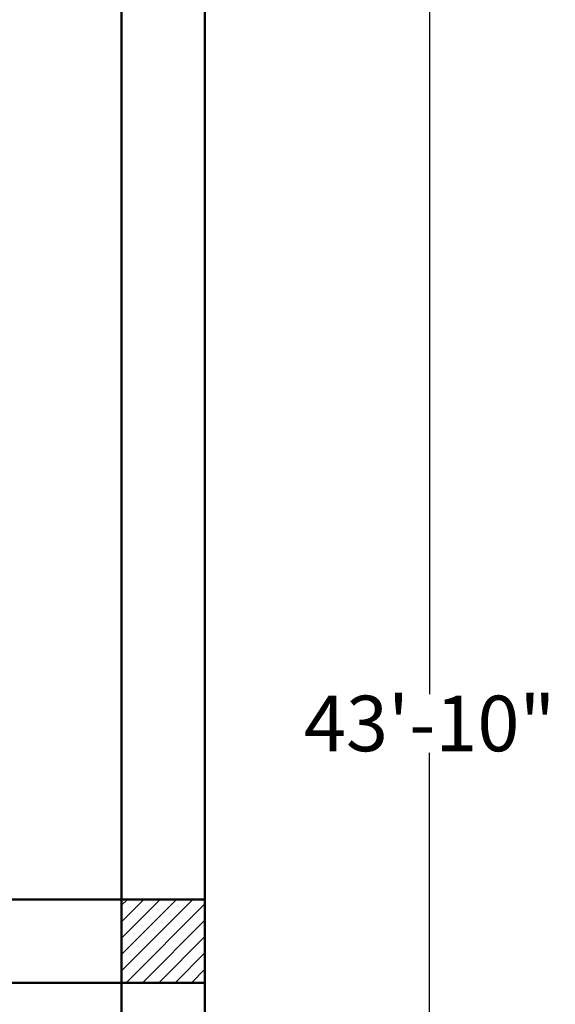
# Model space of a CAD drawing. Units: inches. Extents: x 0 to 281, y -535 to 46.
# Tile 7 of 22: x 223 to 281, y -275 to -168. Entities that reach past the tile are written whole.
import ezdxf

# ---------------------------------------------------------------- set-up
doc = ezdxf.new("R2010")
doc.units = ezdxf.units.IN
doc.header["$MEASUREMENT"] = 0
for name, color, linetype, lineweight in [('A-ANNO-DIMS', 2, 'Continuous', 18), ('A-COLS-PATT', 152, 'Continuous', 13), ('A-WALL', 7, 'Continuous', 50)]:
    doc.layers.add(name, color=color, linetype=linetype, lineweight=lineweight)
doc.styles.get("Standard").update_dxf_attribs({"font": 'arial.ttf'})
doc.dimstyles.get("Standard").update_dxf_attribs({"dimtxt": 0.18, "dimasz": 0.18, "dimexe": 0.18, "dimexo": 0.0625, "dimgap": 0.09, "dimtad": 0, "dimtih": 1, "dimtoh": 1, "dimdec": 0, "dimzin": 0, "dimdsep": 46, "dimlunit": 3, "dimtxsty": 'Standard', "dimcen": 0.09, "dimadec": 0, "dimazin": 0, "dimtfac": 1, "dimtdec": 0, "dimtofl": 0, "dimtmove": 0, "dimatfit": 3, "dimfxl": 1, "dimtolj": 1, "dimtzin": 0, "dimarcsym": 0})

# ---------------------------------------------------------------- blocks, each defined once
blk = doc.blocks.new('*D18')
at = {"layer": 'A-ANNO-DIMS', "color": 0, "lineweight": -2, "transparency": 16777216}
for p, q in [((243.52, 18.59), (267.93, 18.59)), ((267.75, 18.41), (267.75, -241.26)), ((267.75, -507.23), (267.75, -247.57)), ((243.52, -507.41), (267.93, -507.41))]:
    blk.add_line(p, q, dxfattribs=at)
at = {"layer": 'A-ANNO-DIMS', "color": 0, "transparency": 16777216}
for points in [[(267.72, 18.41), (267.78, 18.41), (267.75, 18.59)], [(267.72, -507.23), (267.78, -507.23), (267.75, -507.41)]]:
    blk.add_solid(points, dxfattribs=at)
at = {"layer": 'Defpoints', "color": 0, "transparency": 16777216}
for p in [(243.46, 18.59), (243.46, -507.41), (267.75, -507.41)]:
    blk.add_point(p, dxfattribs=at)
at = {"layer": 'A-ANNO-DIMS', "color": 0, "transparency": 16777216, "insert": (267.75, -244.41), "char_height": 6, "attachment_point": 5}
blk.add_mtext('\\A1;43\'-10"', dxfattribs=at)

msp = doc.modelspace()

# ---------------------------------------------------------------- hatches: boundary and pattern name
at = {"layer": 'A-COLS-PATT'}
h = msp.add_hatch(dxfattribs=at)
h.set_pattern_fill('ANSI31', color=256, scale=10)
h.paths.add_polyline_path([(36.46, 18.59), (27.46, 18.59), (27.46, 9.59), (36.46, 9.59)])
h.paths.add_polyline_path([(165.46, 18.59), (156.46, 18.59), (156.46, 9.59), (165.46, 9.59)])
h.paths.add_polyline_path([(243.46, 18.59), (234.46, 18.59), (234.46, 9.59), (243.46, 9.59)])
h.paths.add_polyline_path([(243.46, -122.41), (234.46, -122.41), (234.46, -131.41), (243.46, -131.41)])
h.paths.add_polyline_path([(36.46, -122.41), (27.46, -122.41), (27.46, -131.41), (36.46, -131.41)])
h.paths.add_polyline_path([(36.46, -498.41), (27.46, -498.41), (27.46, -507.41), (36.46, -507.41)])
h.paths.add_polyline_path([(243.46, -498.41), (234.46, -498.41), (234.46, -507.41), (243.46, -507.41)])
h.paths.add_polyline_path([(159.46, -498.41), (150.46, -498.41), (150.46, -507.41), (159.46, -507.41)])
h.paths.add_polyline_path([(36.46, -392.41), (27.46, -392.41), (27.46, -401.41), (36.46, -401.41)])
h.paths.add_polyline_path([(159.46, -392.41), (150.46, -392.41), (150.46, -401.41), (159.46, -401.41)])
h.paths.add_polyline_path([(243.46, -392.41), (234.46, -392.41), (234.46, -401.41), (243.46, -401.41)])
h.paths.add_polyline_path([(36.46, -263.41), (27.46, -263.41), (27.46, -272.41), (36.46, -272.41)])
h.paths.add_polyline_path([(243.46, -263.41), (234.46, -263.41), (234.46, -272.41), (243.46, -272.41)])

# ---------------------------------------------------------------- linework, layer by layer
at = {"layer": 'A-WALL'}
for p, q in [((234.46, 18.59), (234.46, -507.41)), ((243.46, 18.59), (243.46, -507.41)), ((195.46, -263.41), (243.46, -263.41)), ((195.46, -272.41), (243.46, -272.41))]:
    msp.add_line(p, q, dxfattribs=at)

# ---------------------------------------------------------------- dimensions: what is measured, and where the dimension line sits
at = {"layer": 'A-ANNO-DIMS'}
dim = msp.add_linear_dim(base=(267.75, -507.41), p1=(243.46, 18.59), p2=(243.46, -507.41), angle=90, dimstyle='Standard', override={"dimtxt": 6, "dimclrd": 0, "dimclre": 0, "dimclrt": 0}, dxfattribs=at)
dim.commit()
dim.dimension.update_dxf_attribs({"geometry": '*D18', "text_midpoint": (267.75, -244.41)})

doc.saveas('drawing.dxf')
